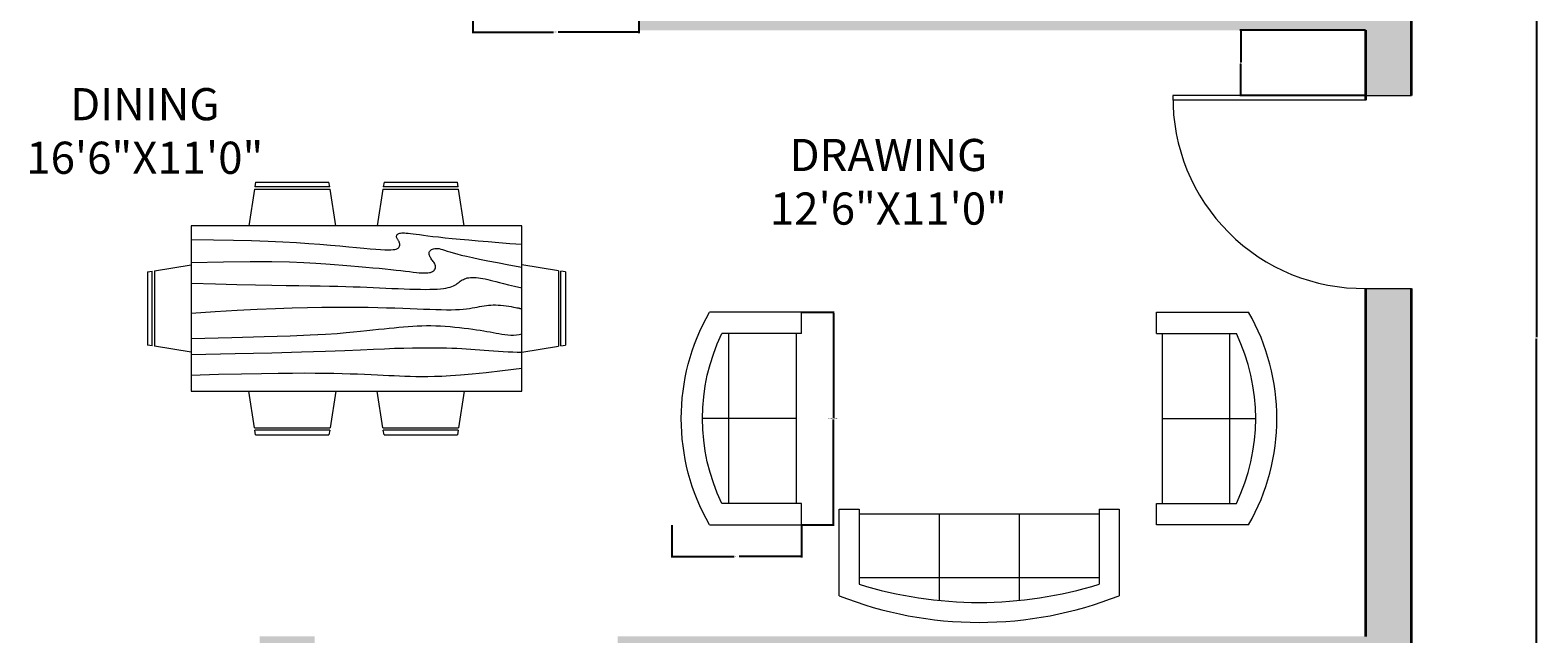
# Model space of a CAD drawing. Units: inches. Extents: x -382 to 250, y 518 to 1732.
# Tile 7 of 8: x -81 to 247, y 1373 to 1504. Entities that reach past the tile are written whole.
import ezdxf

# ---------------------------------------------------------------- set-up
doc = ezdxf.new("R2010")
doc.units = ezdxf.units.IN
doc.header["$MEASUREMENT"] = 0
for name, color, linetype, lineweight in [('A-ANNO-DIMS', 2, 'Continuous', 18), ('A-AREA-IDEN', 7, 'Continuous', 18), ('A-DOOR', 3, 'Continuous', 18), ('A-FURN', 8, 'Continuous', 18), ('A-WALL', 7, 'Continuous', 35)]:
    doc.layers.add(name, color=color, linetype=linetype, lineweight=lineweight)
doc.layers.add('A-WALL-PATT', color=251, linetype='Continuous', lineweight=13, true_color=0x636466)
doc.styles.get("Standard").update_dxf_attribs({"font": 'arial.ttf'})
doc.dimstyles.get("Standard").update_dxf_attribs({"dimtxt": 0.18, "dimasz": 0.18, "dimexe": 0.18, "dimexo": 0.0625, "dimgap": 0.09, "dimtad": 0, "dimtih": 1, "dimtoh": 1, "dimdec": 4, "dimzin": 0, "dimdsep": 46, "dimtxsty": 'Standard', "dimcen": 0.09, "dimadec": 0, "dimazin": 0, "dimtfac": 1, "dimtdec": 4, "dimtofl": 0, "dimtmove": 0, "dimatfit": 3, "dimfxl": 1, "dimtolj": 1, "dimtzin": 0, "dimarcsym": 0})

# ---------------------------------------------------------------- blocks, each defined once
blk = doc.blocks.new('Dining Set - 36 x 72 in.')
for p, q in [((-22, 27.5), (-22.1562, 26.50042)), ((-5.8416, 26.5), (-22.1534, 26.5)), ((-22, 27.5), (-6, 27.5)), ((-5.8437, 26.49966), (-6, 27.5)), ((6, 27.5), (5.8438, 26.50042)), ((22.1584, 26.5), (5.8466, 26.5)), ((6, 27.5), (22, 27.5)), ((22.1563, 26.49966), (22, 27.5)), ((-22.2343, 26.00059), (-23.4847, 17.99762)), ((-22.2304, 26), (-5.7608, 26)), ((-4.5152, 17.99762), (-5.7655, 25.99926)), ((5.7657, 26.00059), (4.5153, 17.99762)), ((5.7696, 26), (22.2392, 26)), ((23.4848, 17.99762), (22.2345, 25.99926)), ((36, 18), (-36, 18)), ((-36, 18), (-36, -18)), ((36, -18), (36, 18)), ((-45.5, 8), (-44.5004, 8.15617)), ((-45.5, 8), (-45.5, -8)), ((-44.5, -8.15843), (-44.5, 8.15338)), ((-44.0006, 8.23428), (-35.9976, 9.48474)), ((-44, 8.23041), (-44, -8.23915)), ((44.0006, 8.23428), (35.9976, 9.48474)), ((44, 8.23041), (44, -8.23915)), ((44.5, -8.15843), (44.5, 8.15338)), ((45.5, 8), (44.5005, 8.15617)), ((45.5, 8), (45.5, -8)), ((-44.4997, -8.15631), (-45.5, -8)), ((-35.9976, -9.48476), (-43.9993, -8.2345)), ((35.9976, -9.48476), (43.9993, -8.2345)), ((44.4997, -8.15631), (45.5, -8)), ((-36, -18), (36, -18)), ((-22.2343, -26.0006), (-23.4847, -17.99762)), ((-4.5152, -17.99762), (-5.7655, -25.99928)), ((5.7657, -26.0006), (4.5153, -17.99762)), ((23.4848, -17.99762), (22.2345, -25.99928)), ((-22.2304, -26), (-5.7608, -26)), ((5.7696, -26), (22.2392, -26)), ((-22, -27.5), (-22.1562, -26.50044)), ((-5.8416, -26.5), (-22.1534, -26.5)), ((-22, -27.5), (-6, -27.5)), ((-5.8437, -26.49967), (-6, -27.5)), ((6, -27.5), (5.8438, -26.50044)), ((22.1584, -26.5), (5.8466, -26.5)), ((6, -27.5), (22, -27.5)), ((22.1563, -26.49967), (22, -27.5))]:
    blk.add_line(p, q)
for points in [[(-36, 15), (-31.1772, 14.97754), (-26.8079, 14.91406), (-22.8538, 14.81543), (-19.276, 14.6875), (-16.0362, 14.53613), (-13.0957, 14.36718), (-10.4159, 14.18652), (-7.9583, 14), (-5.6904, 13.81315), (-3.6035, 13.63021), (-1.6954, 13.45508), (0.0365, 13.29166), (1.5945, 13.14388), (2.9811, 13.01562), (4.1988, 12.9108), (5.25, 12.83333), (6.1393, 12.78613), (6.8802, 12.76823), (7.4883, 12.77767), (7.9792, 12.8125), (8.3685, 12.87077), (8.6719, 12.95052), (8.9049, 13.0498), (9.0833, 13.16666), (9.2205, 13.29899), (9.3216, 13.44401), (9.3895, 13.59879), (9.4271, 13.76041), (9.4373, 13.92594), (9.4232, 14.09245), (9.3875, 14.257), (9.3333, 14.41666), (9.2638, 14.56917), (9.1836, 14.71484), (9.0975, 14.85465), (9.0104, 14.98958), (8.9272, 15.1206), (8.8529, 15.2487), (8.7922, 15.37483), (8.75, 15.5), (8.7305, 15.62467), (8.7344, 15.74739), (8.7617, 15.86621), (8.8125, 15.97916), (8.8867, 16.08431), (8.9844, 16.17968), (9.1055, 16.26334), (9.25, 16.33333), (9.4189, 16.38802), (9.6172, 16.42708), (9.8506, 16.45052), (10.125, 16.45833), (10.4463, 16.45052), (10.8203, 16.42708), (11.2529, 16.38802), (11.75, 16.33333), (12.3184, 16.26318), (12.9694, 16.17838), (13.7151, 16.07991), (14.5677, 15.96875), (15.5395, 15.84586), (16.6426, 15.71224), (17.8893, 15.56884), (19.2917, 15.41666), (20.859, 15.25667), (22.5879, 15.08984), (24.4721, 14.91715), (26.5052, 14.73958), (28.6809, 14.5581), (30.9929, 14.3737), (33.4347, 14.18733), (36, 14)], [(-36, 10), (-28.9766, 10.14274), (-23.1725, 10.20442), (-18.4241, 10.19775), (-14.5677, 10.13541), (-11.4399, 10.03011), (-8.877, 9.89453), (-6.7154, 9.74137), (-4.7917, 9.58333), (-2.9698, 9.43082), (-1.2246, 9.28515), (0.4415, 9.14534), (2.026, 9.01041), (3.5266, 8.87939), (4.9408, 8.7513), (6.266, 8.62516), (7.5, 8.5), (8.6411, 8.37549), (9.6914, 8.2539), (10.6538, 8.13818), (11.5312, 8.03125), (12.3267, 7.93603), (13.043, 7.85547), (13.6831, 7.79248), (14.25, 7.75), (14.7471, 7.7303), (15.1797, 7.73307), (15.5537, 7.75732), (15.875, 7.80208), (16.1494, 7.86637), (16.3828, 7.94922), (16.5811, 8.04964), (16.75, 8.16666), (16.8944, 8.29915), (17.0143, 8.44531), (17.1089, 8.60319), (17.1771, 8.77083), (17.218, 8.94629), (17.2305, 9.1276), (17.2137, 9.31282), (17.1667, 9.5), (17.0895, 9.6875), (16.987, 9.875), (16.8649, 10.0625), (16.7292, 10.25), (16.5856, 10.4375), (16.4401, 10.625), (16.2985, 10.8125), (16.1667, 11), (16.05, 11.18733), (15.9518, 11.3737), (15.8752, 11.5581), (15.8229, 11.73958), (15.798, 11.91715), (15.8034, 12.08984), (15.842, 12.25667), (15.9167, 12.41666), (16.0295, 12.56836), (16.1784, 12.70833), (16.3605, 12.83268), (16.5729, 12.9375), (16.8127, 13.01888), (17.0768, 13.07291), (17.3625, 13.0957), (17.6667, 13.08333), (17.9894, 13.03312), (18.3418, 12.94726), (18.7382, 12.82918), (19.1927, 12.68229), (19.7195, 12.51001), (20.3327, 12.31575), (21.0465, 12.10294), (21.875, 11.875), (22.8357, 11.63354), (23.959, 11.37304), (25.2786, 11.08618), (26.8282, 10.76562), (28.6414, 10.40405), (30.752, 9.99414), (33.1936, 9.52856), (36, 9)], [(-36, 5.5), (-30.7157, 5.3348), (-26.069, 5.20963), (-21.9946, 5.11767), (-18.4271, 5.05208), (-15.3009, 5.00602), (-12.5508, 4.97265), (-10.1112, 4.94515), (-7.9167, 4.91666), (-5.909, 4.88167), (-4.0586, 4.83984), (-2.3429, 4.79215), (-0.7396, 4.73958), (0.7739, 4.6831), (2.22, 4.6237), (3.6213, 4.56233), (5, 4.5), (6.373, 4.43782), (7.7344, 4.3776), (9.0723, 4.32129), (10.375, 4.27083), (11.6309, 4.22819), (12.8281, 4.19531), (13.9551, 4.17415), (15, 4.16666), (15.954, 4.17448), (16.819, 4.19791), (17.6001, 4.23698), (18.3021, 4.29166), (18.9299, 4.36198), (19.4883, 4.44791), (19.9823, 4.54948), (20.4167, 4.66666), (20.7969, 4.79899), (21.1302, 4.94401), (21.4245, 5.09879), (21.6875, 5.26041), (21.9271, 5.42594), (22.1511, 5.59245), (22.3672, 5.757), (22.5834, 5.91666), (22.8065, 6.06868), (23.0404, 6.21093), (23.2879, 6.34147), (23.5521, 6.45833), (23.8358, 6.55957), (24.142, 6.64323), (24.4735, 6.70735), (24.8334, 6.75), (25.2235, 6.76969), (25.642, 6.76692), (26.0858, 6.74267), (26.5521, 6.69791), (27.0379, 6.63362), (27.5404, 6.55078), (28.0565, 6.45036), (28.5834, 6.33333), (29.1242, 6.19987), (29.7071, 6.04687), (30.3661, 5.87044), (31.1354, 5.66666), (32.0493, 5.43164), (33.142, 5.16146), (34.4475, 4.85221), (36, 4.5)], [(-36, -1), (-30.7915, -0.6591), (-26.0195, -0.38216), (-21.6519, -0.16284), (-17.6563, 0.00521), (-14.0005, 0.12833), (-10.6523, 0.21289), (-7.5796, 0.26522), (-4.75, 0.29166), (-2.134, 0.29793), (0.2878, 0.28711), (2.5317, 0.26163), (4.6146, 0.22396), (6.5529, 0.17651), (8.3633, 0.12174), (10.0623, 0.06209), (11.6667, 0), (13.1899, -0.06201), (14.6341, -0.1211), (15.9982, -0.17432), (17.2813, -0.21875), (18.4823, -0.25147), (19.6003, -0.26953), (20.6343, -0.27002), (21.5834, -0.25), (22.4481, -0.20768), (23.2357, -0.14584), (23.9549, -0.06836), (24.6146, 0.02083), (25.2235, 0.11784), (25.7904, 0.21875), (26.3241, 0.31966), (26.8334, 0.41666), (27.3265, 0.50618), (27.8099, 0.58593), (28.2894, 0.65397), (28.7709, 0.70833), (29.2601, 0.74707), (29.763, 0.76823), (30.2855, 0.76985), (30.8334, 0.75), (31.4088, 0.70784), (31.9994, 0.64713), (32.589, 0.57275), (33.1615, 0.48958), (33.7008, 0.4025), (34.1908, 0.3164), (34.6153, 0.23616), (34.9584, 0.16666), (35.2099, 0.11165), (35.3848, 0.07031), (35.504, 0.04069), (35.5886, 0.02083), (35.6594, 0.00879), (35.7377, 0.0026), (35.8442, 0.00032), (36, 0)], [(-36, -6.5), (-27.1843, -6.31267), (-20.084, -6.1263), (-14.469, -5.9419), (-10.1094, -5.76042), (-6.7752, -5.58285), (-4.2363, -5.41016), (-2.2629, -5.24333), (-0.625, -5.08334), (0.8708, -4.93099), (2.2715, -4.78646), (3.5872, -4.64974), (4.8281, -4.52084), (6.0046, -4.39974), (7.127, -4.28646), (8.2053, -4.18099), (9.25, -4.08334), (10.2705, -3.99382), (11.2734, -3.91407), (12.2647, -3.84603), (13.25, -3.79167), (14.2354, -3.75293), (15.2266, -3.73177), (16.2295, -3.73015), (17.25, -3.75), (18.2912, -3.79248), (19.3451, -3.85547), (20.4009, -3.93604), (21.4479, -4.03125), (22.4754, -4.13819), (23.4727, -4.25391), (24.4289, -4.37549), (25.3334, -4.5), (26.1785, -4.62492), (26.9694, -4.74935), (27.7145, -4.87281), (28.4219, -4.99479), (29.1, -5.11483), (29.7572, -5.23242), (30.4016, -5.34709), (31.0417, -5.45834), (31.6837, -5.56437), (32.3262, -5.65821), (32.9658, -5.73153), (33.599, -5.77604), (34.2224, -5.78345), (34.8327, -5.74545), (35.4264, -5.65373), (36, -5.5)], [(-36, -10), (-26.4022, -9.81299), (-18.4675, -9.62891), (-11.9839, -9.45069), (-6.7396, -9.28125), (-2.5226, -9.12354), (0.8789, -8.98047), (3.6769, -8.85498), (6.0833, -8.75), (8.2767, -8.66765), (10.3021, -8.60677), (12.1712, -8.56543), (13.8958, -8.54167), (15.4876, -8.53353), (16.9583, -8.53907), (18.3197, -8.55632), (19.5834, -8.58334), (20.7616, -8.61841), (21.8685, -8.66081), (22.9188, -8.71004), (23.9271, -8.76563), (24.9081, -8.82707), (25.8763, -8.89388), (26.8465, -8.96558), (27.8334, -9.04167), (28.8474, -9.12118), (29.8828, -9.20117), (30.93, -9.27824), (31.9792, -9.34896), (33.0205, -9.40991), (34.0443, -9.45768), (35.0407, -9.48885), (36, -9.5)], [(-36, -14.5), (-30.0881, -14.33513), (-25.0332, -14.21224), (-20.7312, -14.12647), (-17.0781, -14.07292), (-13.97, -14.04671), (-11.3027, -14.04297), (-8.9724, -14.05681), (-6.875, -14.08334), (-4.9224, -14.11833), (-3.0905, -14.16016), (-1.3709, -14.20785), (0.2448, -14.26042), (1.7647, -14.3169), (3.1973, -14.3763), (4.5507, -14.43767), (5.8333, -14.5), (7.0554, -14.5621), (8.235, -14.62175), (9.3922, -14.67652), (10.5469, -14.72396), (11.7192, -14.76164), (12.929, -14.78711), (14.1965, -14.79794), (15.5417, -14.79167), (16.9933, -14.76424), (18.6152, -14.70508), (20.4804, -14.60197), (22.6615, -14.44271), (25.2312, -14.21509), (28.2624, -13.9069), (31.8277, -13.50594), (36, -13)]]:
    blk.add_lwpolyline(points)
blk = doc.blocks.new('Sofa - Roundback 7 ft.')
for p, q in [((-12.00002, -32.4421), (-12.00003, -6.5971)), ((11.99997, -32.4421), (11.99998, -6.5971)), ((-36.000027, -34), (-36.000027, -11.4696)), ((-35.999844, -13.3819), (35.9998, -13.3819)), ((35.99998, -34), (35.99998, -11.4696)), ((-36.000027, -32.4421), (35.99998, -32.4421))]:
    blk.add_line(p, q)
for points in [[(-36.000027, -34), (-42.000027, -34), (-42.000027, -8)], [(41.99998, -8), (41.99998, -34), (35.99998, -34)]]:
    blk.add_lwpolyline(points)
for centre, radius, start, end in [((0, -114.25), 114.25, 68.43141, 111.5686), ((-0.00001, -127.1968), 121.1968, 72.72033, 107.2797)]:
    blk.add_arc(centre, radius, start, end)
blk = doc.blocks.new('Sofa - Roundback Loveseat 5 ft.')
for p, q in [((0, -32.44198), (0, -5.99998)), ((-24, -33.99998), (-24, -11.46958)), ((24.00004, -33.99998), (24.00004, -11.46958)), ((-23.9998, -13.38178), (23.99986, -13.38178)), ((-24, -32.44198), (24.00004, -32.44198))]:
    blk.add_line(p, q)
for points in [[(-24, -33.99998), (-30, -33.99998), (-30, -7.99998)], [(30.00004, -7.99998), (30.00004, -33.99998), (24.00004, -33.99998)]]:
    blk.add_lwpolyline(points)
for centre, radius, start, end in [((0, -60.24998), 60.24998, 60.13715, 119.8628), ((0, -61.38438), 55.38444, 64.32083, 115.6792)]:
    blk.add_arc(centre, radius, start, end)
blk = doc.blocks.new('DOOR-ENTRY-42IN')
for p, q in [((0, 0), (-42, 0)), ((0, -1), (-42, -1))]:
    blk.add_line(p, q)
blk.add_arc((-0.5, -0.5), 41.5, 179.3097, 270.6903)
blk = doc.blocks.new('*D32')
at = {"layer": 'A-ANNO-DIMS', "color": 0, "lineweight": -2, "transparency": 16777216}
for p, q in [((86.94, 1442.63), (94, 1442.63)), ((93.82, 1442.45), (93.82, 1419.68)), ((93.82, 1396.55), (93.82, 1419.32)), ((86.94, 1396.37), (94, 1396.37))]:
    blk.add_line(p, q, dxfattribs=at)
at = {"layer": 'A-ANNO-DIMS', "color": 0, "transparency": 16777216}
for points in [[(93.79, 1442.45), (93.85, 1442.45), (93.82, 1442.63)], [(93.79, 1396.55), (93.85, 1396.55), (93.82, 1396.37)]]:
    blk.add_solid(points, dxfattribs=at)
at = {"layer": 'Defpoints', "color": 0, "transparency": 16777216}
for p in [(86.88, 1442.63), (86.88, 1396.37), (93.82, 1396.37)]:
    blk.add_point(p, dxfattribs=at)
at = {"layer": 'A-ANNO-DIMS', "color": 0, "transparency": 16777216, "insert": (93.82, 1419.5), "char_height": 0.18, "attachment_point": 5}
blk.add_mtext('\\A1;LOVESEAT 46 TYP.', dxfattribs=at)
blk = doc.blocks.new('*D33')
at = {"layer": 'A-ANNO-DIMS', "color": 0, "lineweight": -2, "transparency": 16777216}
for p, q in [((58.61, 1396.31), (58.61, 1389.26)), ((86.88, 1396.31), (86.88, 1389.26)), ((58.79, 1389.44), (72.21, 1389.44)), ((86.7, 1389.44), (73.27, 1389.44))]:
    blk.add_line(p, q, dxfattribs=at)
at = {"layer": 'A-ANNO-DIMS', "color": 0, "transparency": 16777216}
for points in [[(58.79, 1389.47), (58.79, 1389.41), (58.61, 1389.44)], [(86.7, 1389.47), (86.7, 1389.41), (86.88, 1389.44)]]:
    blk.add_solid(points, dxfattribs=at)
at = {"layer": 'Defpoints', "color": 0, "transparency": 16777216}
for p in [(58.61, 1396.37), (86.88, 1396.37), (58.61, 1389.44)]:
    blk.add_point(p, dxfattribs=at)
at = {"layer": 'A-ANNO-DIMS', "color": 0, "transparency": 16777216, "insert": (72.74, 1389.44), "char_height": 0.18, "attachment_point": 5}
blk.add_mtext('\\A1;28 TYP.', dxfattribs=at)
blk = doc.blocks.new('*D63')
at = {"layer": 'A-ANNO-DIMS', "color": 0, "lineweight": -2, "transparency": 16777216}
for p, q in [((15.29, 1509.01), (15.29, 1503.44)), ((51.42, 1509.01), (51.42, 1503.44)), ((15.47, 1503.62), (32.82, 1503.62)), ((51.24, 1503.62), (33.88, 1503.62))]:
    blk.add_line(p, q, dxfattribs=at)
at = {"layer": 'A-ANNO-DIMS', "color": 0, "transparency": 16777216}
for points in [[(15.47, 1503.65), (15.47, 1503.59), (15.29, 1503.62)], [(51.24, 1503.65), (51.24, 1503.59), (51.42, 1503.62)]]:
    blk.add_solid(points, dxfattribs=at)
at = {"layer": 'Defpoints', "color": 0, "transparency": 16777216}
for p in [(15.29, 1509.07), (51.42, 1509.07), (51.42, 1503.62)]:
    blk.add_point(p, dxfattribs=at)
at = {"layer": 'A-ANNO-DIMS', "color": 0, "transparency": 16777216, "insert": (33.35, 1503.62), "char_height": 0.18, "attachment_point": 5}
blk.add_mtext('\\A1;36 TYP.', dxfattribs=at)
blk = doc.blocks.new('*D87')
at = {"layer": 'A-ANNO-DIMS', "color": 0, "lineweight": -2, "transparency": 16777216}
for p, q in [((87.85, 1704.87), (247.16, 1704.87)), ((246.98, 1704.69), (246.98, 1437.22)), ((246.98, 1169.38), (246.98, 1436.85)), ((82.25, 1169.2), (247.16, 1169.2))]:
    blk.add_line(p, q, dxfattribs=at)
at = {"layer": 'A-ANNO-DIMS', "color": 0, "transparency": 16777216}
for points in [[(246.95, 1704.69), (247.01, 1704.69), (246.98, 1704.87)], [(246.95, 1169.38), (247.01, 1169.38), (246.98, 1169.2)]]:
    blk.add_solid(points, dxfattribs=at)
at = {"layer": 'Defpoints', "color": 0, "transparency": 16777216}
for p in [(87.78, 1704.87), (246.98, 1704.87), (82.19, 1169.2)]:
    blk.add_point(p, dxfattribs=at)
at = {"layer": 'A-ANNO-DIMS', "color": 0, "transparency": 16777216, "insert": (246.98, 1437.03), "char_height": 0.18, "attachment_point": 5}
blk.add_mtext('\\A1;535.7', dxfattribs=at)
blk = doc.blocks.new('*D95')
at = {"layer": 'A-ANNO-DIMS', "color": 0, "lineweight": -2, "transparency": 16777216}
for p, q in [((209.72, 1504.07), (182.4, 1504.07)), ((182.58, 1503.89), (182.58, 1497.13)), ((182.58, 1490.01), (182.58, 1496.77)), ((209.72, 1489.83), (182.4, 1489.83))]:
    blk.add_line(p, q, dxfattribs=at)
at = {"layer": 'A-ANNO-DIMS', "color": 0, "transparency": 16777216}
for points in [[(182.55, 1503.89), (182.61, 1503.89), (182.58, 1504.07)], [(182.55, 1490.01), (182.61, 1490.01), (182.58, 1489.83)]]:
    blk.add_solid(points, dxfattribs=at)
at = {"layer": 'Defpoints', "color": 0, "transparency": 16777216}
for p in [(182.58, 1504.07), (209.78, 1504.07), (209.78, 1489.83)]:
    blk.add_point(p, dxfattribs=at)
at = {"layer": 'A-ANNO-DIMS', "color": 0, "transparency": 16777216, "insert": (182.58, 1496.95), "char_height": 0.18, "attachment_point": 5}
blk.add_mtext('\\A1;14.234', dxfattribs=at)

msp = doc.modelspace()

# ---------------------------------------------------------------- hatches: boundary and pattern name
at = {"layer": 'A-WALL-PATT'}
h = msp.add_hatch(color=256, dxfattribs=at)
h.dxf.hatch_style = 1
h.paths.add_polyline_path([(219.785, 1529.2079), (209.785, 1529.2079), (209.785, 1509.0687), (51.2853, 1509.0687), (51.2853, 1504.0687), (209.785, 1504.0687), (209.785, 1489.835), (219.785, 1489.835)])
h = msp.add_hatch(color=256, dxfattribs=at)
h.dxf.hatch_style = 1
h.paths.add_polyline_path([(219.785, 1367.0687), (219.785, 1447.835), (209.785, 1447.835), (209.785, 1372.0687), (46.785, 1372.0687), (46.785, 1367.0687), (209.785, 1367.0687), (209.785, 1272.0687), (125.7302, 1272.0687), (125.7302, 1267.0687), (209.785, 1267.0687), (209.785, 1207.0687), (56.785, 1207.0687), (56.785, 1267.0687), (89.7302, 1267.0687), (89.7302, 1272.0687), (56.785, 1272.0687), (56.785, 1314.0687), (-19.215, 1314.0687), (-19.215, 1372.0687), (-31.1575, 1372.0687), (-31.1575, 1367.0687), (-24.215, 1367.0687), (-24.215, 1304.7972), (-19.215, 1304.7972), (-19.215, 1309.0687), (46.785, 1309.0687), (46.785, 1207.0687), (17.0948, 1207.0687), (17.0948, 1197.0687), (56.7186, 1197.0687), (219.785, 1197.0687)])

# ---------------------------------------------------------------- linework, layer by layer
at = {"layer": 'A-DOOR'}
for p, q in [((209.785, 1489.835), (219.785, 1489.835)), ((209.785, 1447.835), (219.785, 1447.835))]:
    msp.add_line(p, q, dxfattribs=at)
at = {"layer": 'A-WALL'}
for p, q in [((219.785, 1489.835), (219.785, 1663.0687)), ((209.785, 1488.835), (209.785, 1504.0687)), ((209.785, 1372.0687), (209.785, 1447.835)), ((219.785, 1367.0687), (219.785, 1447.835))]:
    msp.add_line(p, q, dxfattribs=at)

# ---------------------------------------------------------------- block references
at = {"layer": 'A-DOOR'}
msp.add_blockref('DOOR-ENTRY-42IN', (209.785, 1489.835), dxfattribs=at)
at = {"layer": 'A-FURN'}
msp.add_blockref('Dining Set - 36 x 72 in.', (-10.0845, 1443.4625), dxfattribs=at)
for name, p, xscale, yscale, zscale, rotation in [('Sofa - Roundback Loveseat 5 ft.', (60.6669, 1419.5016), -0.7709074640759157, 0.7709074640759157, 0.7709074640759157, 90.00001000000114), ('Sofa - Roundback Loveseat 5 ft.', (190.4468, 1419.5016), 0.7709074640759157, 0.7709074640759157, 0.7709074640759157, 270), ('Sofa - Roundback 7 ft.', (125.5568, 1375.1056), 0.7259645452068219, 0.7259645452068219, 0.7259645452068219, 179.9999999999999)]:
    msp.add_blockref(name, p, dxfattribs=dict(at, xscale=xscale, yscale=yscale, zscale=zscale, rotation=rotation))

# ---------------------------------------------------------------- texts
at = {"layer": 'A-AREA-IDEN', "char_height": 7, "attachment_point": 1}
for s, insert in [('\\pxqc;DINING\\P16\'6"X11\'0"', (-96.0331, 1491.4558)), ('\\pxqc;DRAWING\\P12\'6"X11\'0"', (65.9707, 1480.3899))]:
    msp.add_mtext_dynamic_manual_height_columns(s, width=79.656175, gutter_width=1, heights=[0], dxfattribs=dict(at, insert=insert))

# ---------------------------------------------------------------- dimensions: what is measured, and where the dimension line sits
at = {"layer": 'A-ANNO-DIMS'}
for base, p1, p2, override, picture, middle in [((246.985, 1704.8705), (82.1869, 1169.1977), (87.785, 1704.8705), {"dimdec": 1, "dimlfac": 1, "dimrnd": 0, "dimzin": 0, "dimdsep": 46, "dimlunit": 2}, '*D87', (246.985, 1437.0341)), ((182.585, 1504.0687), (209.785, 1489.835), (209.785, 1504.0687), {"dimdec": 3, "dimlfac": 1, "dimrnd": 0, "dimzin": 0, "dimdsep": 46, "dimlunit": 2}, '*D95', (182.585, 1496.9518))]:
    dim = msp.add_linear_dim(base=base, p1=p1, p2=p2, angle=90, dimstyle='Standard', override=override, dxfattribs=at)
    dim.commit()
    dim.dimension.update_dxf_attribs({"geometry": picture, "text_midpoint": middle})
dim = msp.add_linear_dim(base=(51.4204, 1503.6159), p1=(15.2853, 1509.0687), p2=(51.4204, 1509.0687), text='<> TYP.', dimstyle='Standard', override={"dimdec": 0, "dimlfac": 1, "dimrnd": 0, "dimzin": 0, "dimdsep": 46, "dimlunit": 2}, dxfattribs=at)
dim.commit()
dim.dimension.update_dxf_attribs({"geometry": '*D63', "text_midpoint": (33.3528, 1503.6159)})
for base, p1, p2, angle, text, picture, middle in [((93.816, 1396.3743), (86.8778, 1442.6288), (86.8778, 1396.3743), 270.00001, 'LOVESEAT <> TYP.', '*D32', (93.816, 1419.5016)), ((58.6112, 1389.4362), (86.8778, 1396.3743), (58.6112, 1396.3743), 180.00001, '<> TYP.', '*D33', (72.7445, 1389.4362))]:
    dim = msp.add_linear_dim(base=base, p1=p1, p2=p2, angle=angle, text=text, dimstyle='Standard', override={"dimdec": 0, "dimlfac": 1, "dimrnd": 0, "dimzin": 0, "dimdsep": 46, "dimlunit": 2}, dxfattribs=at)
    dim.commit()
    dim.dimension.update_dxf_attribs({"geometry": picture, "text_midpoint": middle})

doc.saveas('drawing.dxf')
